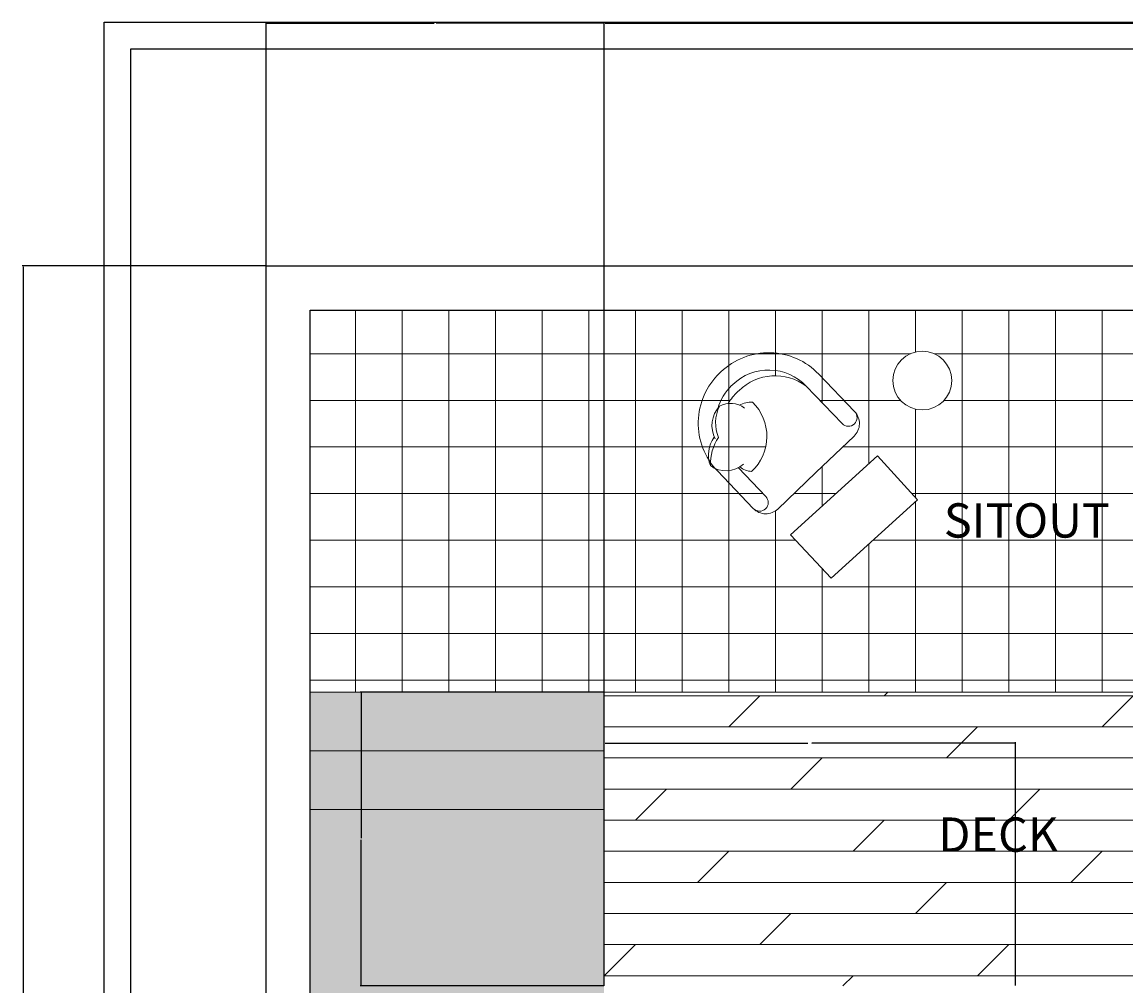
# Model space of a CAD drawing. Units: inches. Extents: x 84 to 1044, y -280 to 906.
# Tile 51 of 105: x 84 to 310, y 709 to 906. Entities that reach past the tile are written whole.
import ezdxf

# ---------------------------------------------------------------- set-up
doc = ezdxf.new("R2010")
doc.units = ezdxf.units.IN
for name, color, linetype, lineweight in [('A-ANNO-DIMS', 2, 'Continuous', 18), ('A-ANNO-TTLB', 7, 'Continuous', 25), ('A-AREA-IDEN', 7, 'Continuous', 13), ('A-FURN', 8, 'Continuous', 15), ('A-STAIRCASE', 144, 'Continuous', 18), ('C-PROP', 7, 'Continuous', 25), ('L-HRDS', 32, 'Continuous', 18)]:
    doc.layers.add(name, color=color, linetype=linetype, lineweight=lineweight)
for name, color, linetype, lineweight, true_color in [('A-FLOR-PATT', 251, 'Continuous', 9, 0x705861), ('A-FLOR-STRS-PATT', 35, 'Continuous', 9, 0x947764), ('L-PLNT-PATT', 9, 'Continuous', 9, 0xafd9aa)]:
    doc.layers.add(name, color=color, linetype=linetype, lineweight=lineweight, true_color=true_color)
doc.styles.add('1-100DIM', font='txt', dxfattribs={"height": 0.3})
doc.styles.get("Standard").update_dxf_attribs({"font": 'arial.ttf'})
doc.dimstyles.get("Standard").update_dxf_attribs({"dimtxt": 0.18, "dimasz": 0.18, "dimexe": 0.18, "dimexo": 0.0625, "dimgap": 0.09, "dimtad": 0, "dimtih": 1, "dimtoh": 1, "dimdec": 4, "dimzin": 0, "dimdsep": 46, "dimtxsty": 'Standard', "dimcen": 0.09, "dimadec": 0, "dimazin": 0, "dimtfac": 1, "dimtdec": 4, "dimtofl": 0, "dimtmove": 0, "dimatfit": 3, "dimfxl": 1, "dimtolj": 1, "dimtzin": 0, "dimarcsym": 0})

# ---------------------------------------------------------------- blocks, each defined once
blk = doc.blocks.new('*D61')
at = {"layer": 'A-ANNO-DIMS', "color": 0, "lineweight": -2, "transparency": 16777216}
for p, q in [((134.12, 856.12), (84.4, 856.12)), ((84.58, 855.94), (84.58, 367.3)), ((84.58, -121.7), (84.58, 366.94)), ((134.12, -121.88), (84.4, -121.88))]:
    blk.add_line(p, q, dxfattribs=at)
at = {"layer": 'A-ANNO-DIMS', "color": 0, "transparency": 16777216}
for points in [[(84.55, 855.94), (84.61, 855.94), (84.58, 856.12)], [(84.55, -121.7), (84.61, -121.7), (84.58, -121.88)]]:
    blk.add_solid(points, dxfattribs=at)
at = {"layer": 'Defpoints', "color": 0, "transparency": 16777216}
for p in [(84.58, 856.12), (134.18, 856.12), (134.18, -121.88)]:
    blk.add_point(p, dxfattribs=at)
at = {"layer": 'A-ANNO-DIMS', "color": 0, "transparency": 16777216, "insert": (84.58, 367.12), "char_height": 0.18, "attachment_point": 5}
blk.add_mtext('\\A1;978', dxfattribs=at)
blk = doc.blocks.new('*D62')
at = {"layer": 'A-ANNO-DIMS', "color": 0, "lineweight": -2, "transparency": 16777216}
for p, q in [((203.18, 709.18), (203.18, 905.9)), ((896.07, 400.18), (896.07, 905.9)), ((203.36, 905.72), (549.23, 905.72)), ((895.89, 905.72), (550.02, 905.72))]:
    blk.add_line(p, q, dxfattribs=at)
at = {"layer": 'A-ANNO-DIMS', "color": 0, "transparency": 16777216}
for points in [[(203.36, 905.75), (203.36, 905.69), (203.18, 905.72)], [(895.89, 905.75), (895.89, 905.69), (896.07, 905.72)]]:
    blk.add_solid(points, dxfattribs=at)
at = {"layer": 'Defpoints', "color": 0, "transparency": 16777216}
for p in [(896.07, 905.72), (203.18, 709.12), (896.07, 400.12)]:
    blk.add_point(p, dxfattribs=at)
at = {"layer": 'A-ANNO-DIMS', "color": 0, "transparency": 16777216, "insert": (549.63, 905.72), "char_height": 0.18, "attachment_point": 5}
blk.add_mtext('\\A1;692.9', dxfattribs=at)
blk = doc.blocks.new('*D64')
at = {"layer": 'A-ANNO-DIMS', "color": 0, "lineweight": -2, "transparency": 16777216}
for p, q in [((134.18, 856.18), (134.18, 905.9)), ((203.18, 709.18), (203.18, 905.9)), ((134.36, 905.72), (168.46, 905.72)), ((203, 905.72), (168.9, 905.72))]:
    blk.add_line(p, q, dxfattribs=at)
at = {"layer": 'A-ANNO-DIMS', "color": 0, "transparency": 16777216}
for points in [[(134.36, 905.75), (134.36, 905.69), (134.18, 905.72)], [(203, 905.75), (203, 905.69), (203.18, 905.72)]]:
    blk.add_solid(points, dxfattribs=at)
at = {"layer": 'Defpoints', "color": 0, "transparency": 16777216}
for p in [(203.18, 905.72), (134.18, 856.12), (203.18, 709.12)]:
    blk.add_point(p, dxfattribs=at)
at = {"layer": 'A-ANNO-DIMS', "color": 0, "transparency": 16777216, "insert": (168.68, 905.72), "char_height": 0.18, "attachment_point": 5}
blk.add_mtext('\\A1;69', dxfattribs=at)
blk = doc.blocks.new('*D77')
at = {"layer": 'A-ANNO-DIMS', "color": 0, "lineweight": -2, "transparency": 16777216}
for p, q in [((203.18, 709.18), (203.18, 758.9)), ((203.36, 758.72), (244.76, 758.72)), ((286.95, 758.72), (245.55, 758.72)), ((287.13, 709.18), (287.13, 758.9))]:
    blk.add_line(p, q, dxfattribs=at)
at = {"layer": 'A-ANNO-DIMS', "color": 0, "transparency": 16777216}
for points in [[(203.36, 758.75), (203.36, 758.69), (203.18, 758.72)], [(286.95, 758.75), (286.95, 758.69), (287.13, 758.72)]]:
    blk.add_solid(points, dxfattribs=at)
at = {"layer": 'Defpoints', "color": 0, "transparency": 16777216}
for p in [(287.13, 758.72), (203.18, 709.12), (287.13, 709.12)]:
    blk.add_point(p, dxfattribs=at)
at = {"layer": 'A-ANNO-DIMS', "color": 0, "transparency": 16777216, "insert": (245.15, 758.72), "char_height": 0.18, "attachment_point": 5}
blk.add_mtext('\\A1;83.95', dxfattribs=at)
blk = doc.blocks.new('*D78')
at = {"layer": 'A-ANNO-DIMS', "color": 0, "lineweight": -2, "transparency": 16777216}
for p, q in [((203.12, 769.12), (153.4, 769.12)), ((153.58, 768.94), (153.58, 739.3)), ((153.58, 709.3), (153.58, 738.94)), ((203.12, 709.12), (153.4, 709.12))]:
    blk.add_line(p, q, dxfattribs=at)
at = {"layer": 'A-ANNO-DIMS', "color": 0, "transparency": 16777216}
for points in [[(153.55, 768.94), (153.61, 768.94), (153.58, 769.12)], [(153.55, 709.3), (153.61, 709.3), (153.58, 709.12)]]:
    blk.add_solid(points, dxfattribs=at)
at = {"layer": 'Defpoints', "color": 0, "transparency": 16777216}
for p in [(153.58, 769.12), (203.18, 769.12), (203.18, 709.12)]:
    blk.add_point(p, dxfattribs=at)
at = {"layer": 'A-ANNO-DIMS', "color": 0, "transparency": 16777216, "insert": (153.58, 739.12), "char_height": 0.18, "attachment_point": 5}
blk.add_mtext('\\A1;60', dxfattribs=at)

msp = doc.modelspace()

# ---------------------------------------------------------------- hatches: boundary and pattern name
at = {"layer": 'A-FLOR-PATT', "transparency": 33554597}
h = msp.add_hatch(dxfattribs=at)
h.set_pattern_fill('ANSI37', color=256, scale=3, angle=45)
h.paths.add_polyline_path([(410.074, 847.12), (143.179, 847.12), (143.179, 769.12), (203.179, 769.12), (410.074, 769.12)])
h.paths.add_polyline_path([(254.313, 826.374, -0.4142136), (254.257, 823.878, -0.4142136), (251.76, 823.934), (244.439, 831.592, 0.3775004), (230.555, 830.526, 0.0765992), (228.51, 828.052, -0.127919), (230.803, 827.709, -0.1215233), (233.469, 828.328, -0.4259892), (233.291, 814.163, -0.1655406), (230.889, 815.094, -0.0168883), (230.578, 814.914), (236.189, 809.046, -0.4142136), (236.133, 806.549, -0.4142136), (233.636, 806.605, 0.4142136), (238.63, 806.493), (246.415, 813.937), (254.201, 821.381, 0.4142136)], flags=16)
h.paths.add_polyline_path([(241.241, 801.211), (258.998, 817.357), (267.168, 808.372), (249.545, 792.347)], flags=16)
h.paths.add_polyline_path([(262.121, 832.717, -1), (274.121, 832.717, -1)], flags=16)
h.paths.add_polyline_path([(315.269, 832.717, -1), (327.269, 832.717, -1)], flags=16)
h.paths.add_polyline_path([(322.221, 808.372), (330.392, 817.357), (348.148, 801.211), (339.844, 792.347)], flags=16)
h.paths.add_polyline_path([(344.951, 831.592, -0.3727189), (358.711, 830.652), (358.966, 830.408, -0.0723842), (360.879, 828.052, -0.1030417), (362.667, 827.476, -0.0234196), (363.022, 827.039, 0.1348317), (360.058, 831.805, 0.4191038)], flags=0)
h.paths.add_polyline_path([(355.753, 806.605, -0.4142136), (353.257, 806.549, -0.4142136), (353.201, 809.046), (358.811, 814.914, 0.2341585), (363.536, 814.769, 0.4037218), (362.499, 834.358, 0.4178796), (342.398, 834.032), (335.076, 826.374, 0.4142136), (335.188, 821.381), (342.974, 813.937), (350.76, 806.493, 0.4142136)], flags=16)
h = msp.add_hatch(dxfattribs=at)
h.set_pattern_fill('DOLMIT', color=256)
h.paths.add_polyline_path([(896.074, 709.12), (833.074, 709.12), (833.074, 646.12), (833.074, 574.12), (833.074, 511.12), (896.074, 511.12)])
h.paths.add_polyline_path([(386.074, 769.12), (203.179, 769.12), (203.179, 709.12), (287.127, 709.12), (359.127, 709.12), (386.074, 709.12)])
at = {"layer": 'A-FLOR-STRS-PATT', "transparency": 33554567}
h = msp.add_hatch(color=256, dxfattribs=at)
h.dxf.hatch_style = 1
h.paths.add_polyline_path([(650.074, 91.12), (638.074, 91.12), (638.074, 67.12), (455.074, 67.12), (455.074, 55.12), (650.074, 55.12)], flags=17)
h.paths.add_polyline_path([(662.074, 91.12), (650.074, 91.12), (650.074, 55.12), (455.074, 55.12), (455.074, 43.12), (662.074, 43.12)])
h.paths.add_polyline_path([(674.074, 91.12), (671.074, 91.12), (662.074, 91.12), (662.074, 43.12), (455.074, 43.12), (455.074, 31.12), (674.074, 31.12)])
h.paths.add_polyline_path([(227.179, 151.12), (203.179, 151.12), (143.179, 151.12), (143.179, 139.12), (227.179, 139.12)])
h.paths.add_polyline_path([(227.179, 139.12), (143.179, 139.12), (143.179, 127.12), (227.179, 127.12)])
h.paths.add_polyline_path([(203.179, 271.12), (143.179, 271.12), (143.179, 259.12), (203.179, 259.12)])
h.paths.add_polyline_path([(203.179, 259.12), (143.179, 259.12), (143.179, 247.12), (203.179, 247.12)])
h.paths.add_polyline_path([(203.179, 769.12), (143.179, 769.12), (143.179, 757.12), (203.179, 757.12)])
h.paths.add_polyline_path([(203.179, 757.12), (143.179, 757.12), (143.179, 745.12), (203.179, 745.12)])
h.paths.add_polyline_path([(434.074, 847.12), (422.074, 847.12), (422.074, 769.12), (434.074, 769.12)])
h.paths.add_polyline_path([(422.074, 847.12), (410.074, 847.12), (410.074, 769.12), (422.074, 769.12)])
at = {"layer": 'L-PLNT-PATT', "transparency": 33554597}
h = msp.add_hatch(color=256, dxfattribs=at)
h.dxf.hatch_style = 1
h.paths.add_polyline_path([(434.074, 769.12), (386.074, 769.12), (386.074, 709.12), (434.074, 709.12)])
h.paths.add_polyline_path([(896.074, 847.12), (434.074, 847.12), (434.074, 769.12), (434.074, 709.12), (470.074, 709.12), (506.074, 709.12), (572.074, 709.12), (608.074, 709.12), (698.074, 709.12), (770.074, 709.12), (833.074, 709.12), (896.074, 709.12)])
h.paths.add_polyline_path([(983.074, 847.12), (896.074, 847.12), (896.074, 709.12), (896.074, 547.12), (932.074, 547.12), (983.074, 547.12)])
h.paths.add_polyline_path([(983.074, 547.12), (932.074, 547.12), (932.074, 265.12), (983.074, 265.12)])
h.paths.add_polyline_path([(203.179, 646.12), (203.179, 709.12), (203.179, 745.12), (143.179, 745.12), (143.179, 271.12), (203.179, 271.12), (203.179, 274.12), (203.179, 310.12), (203.179, 574.12)])

# ---------------------------------------------------------------- linework, layer by layer
at = {"layer": 'A-ANNO-TTLB'}
for points in [[(101.1, 905.916), (1027.308, 905.916), (1027.308, -279.764), (101.1, -279.764)], [(106.576, 900.439), (1021.832, 900.439), (1021.832, -274.288), (106.576, -274.288)]]:
    msp.add_lwpolyline(points, close=True, dxfattribs=at)
at = {"layer": 'A-FURN'}
for points in [[(246.415, 813.937), (254.201, 821.381, 0.4142136), (254.313, 826.374), (246.991, 834.032, 0.4142136), (227.018, 834.481), (226.89, 834.359), (226.763, 834.237, 0.4142136), (226.314, 814.263), (233.636, 806.605, 0.4142136), (238.63, 806.493), (246.415, 813.937)], [(244.439, 831.592, 0.4142136), (229.459, 831.928), (229.331, 831.806)], [(244.439, 831.592, 0.3727189), (230.679, 830.652), (230.551, 830.53)], [(226.368, 827.039, -0.1305915), (229.203, 831.684), (229.331, 831.806)], [(244.438, 831.592), (251.76, 823.934, 0.4142136), (254.257, 823.878), (254.257, 823.878, 0.4142136), (254.313, 826.374)], [(228.51, 828.052, -0.0723842), (230.424, 830.408), (230.551, 830.53)], [(224.874, 815.352, -0.1477299), (226.507, 821.112, -0.2133428), (226.722, 827.476, -0.1786618)], [(225.824, 820.794, -0.3066635), (226.722, 827.476, -0.30633), (231.866, 827.076, 0.8728472)], [(230.889, 815.094, 0.1655406), (233.291, 814.163, 0.4259892), (233.469, 828.328, 0.1215233), (230.803, 827.709, -7.1154643)], [(231.607, 815.632, -0.3567724), (224.874, 815.352, -0.2495421), (225.653, 821.172, 9.6168803)], [(230.578, 814.914), (236.189, 809.046, -0.4142136), (236.133, 806.549), (236.133, 806.549, -0.4142136), (233.636, 806.605)]]:
    msp.add_lwpolyline(points, format="xyb", dxfattribs=at)
msp.add_lwpolyline([(258.998, 817.357), (267.168, 808.372), (249.545, 792.347), (241.241, 801.211)], close=True, dxfattribs=at)
msp.add_circle((268.121, 832.717), 6, dxfattribs=at)
at = {"layer": 'A-STAIRCASE'}
for p, q in [((203.179, 769.12), (143.179, 769.12)), ((203.179, 757.12), (143.179, 757.12)), ((203.179, 745.12), (143.179, 745.12))]:
    msp.add_line(p, q, dxfattribs=at)
at = {"layer": 'C-PROP'}
for points in [[(143.179, -121.88), (134.179, -121.88), (134.179, 856.12), (992.074, 856.12), (992.074, -121.88), (624.574, -121.88)], [(143.179, -112.88), (143.179, 847.12), (983.074, 847.12), (983.074, -112.88), (624.574, -112.88)]]:
    msp.add_lwpolyline(points, dxfattribs=at)
at = {"layer": 'L-HRDS'}
for p, q in [((203.179, 709.12), (203.179, 769.12)), ((203.179, 769.12), (434.074, 769.12))]:
    msp.add_line(p, q, dxfattribs=at)

# ---------------------------------------------------------------- texts
at = {"layer": 'A-AREA-IDEN', "char_height": 7, "attachment_point": 1, "style": '1-100DIM'}
for s, insert in [('{\\f@Malgun Gothic|b0|i0|c0|p34; SITOUT }', (270.387, 807.659)), ('{\\f@Malgun Gothic|b0|i0|c0|p34;    DECK }', (262.833, 743.516))]:
    msp.add_mtext_dynamic_manual_height_columns(s, width=51.07953, gutter_width=15.851, heights=[0], dxfattribs=dict(at, insert=insert))

# ---------------------------------------------------------------- dimensions: what is measured, and where the dimension line sits
at = {"layer": 'A-ANNO-DIMS'}
for base, p1, p2, override, picture, middle in [((203.179, 905.72), (134.179, 856.12), (203.179, 709.12), {"dimdec": 0, "dimlfac": 1, "dimrnd": 0, "dimzin": 0, "dimdsep": 46, "dimlunit": 2}, '*D64', (168.679, 905.72)), ((896.074, 905.72), (203.179, 709.12), (896.074, 400.12), {"dimdec": 1, "dimlfac": 1, "dimrnd": 0, "dimzin": 0, "dimdsep": 46, "dimlunit": 2}, '*D62', (549.627, 905.72)), ((287.127, 758.72), (203.179, 709.12), (287.127, 709.12), {"dimdec": 2, "dimlfac": 1, "dimrnd": 0, "dimzin": 0, "dimdsep": 46, "dimlunit": 2}, '*D77', (245.153, 758.72))]:
    dim = msp.add_linear_dim(base=base, p1=p1, p2=p2, dimstyle='Standard', override=override, dxfattribs=at)
    dim.commit()
    dim.dimension.update_dxf_attribs({"geometry": picture, "text_midpoint": middle})
for base, p1, p2, picture, middle in [((84.579, 856.12), (134.179, -121.88), (134.179, 856.12), '*D61', (84.579, 367.12)), ((153.579, 769.12), (203.179, 709.12), (203.179, 769.12), '*D78', (153.579, 739.12))]:
    dim = msp.add_linear_dim(base=base, p1=p1, p2=p2, angle=90, dimstyle='Standard', override={"dimdec": 0, "dimlfac": 1, "dimrnd": 0, "dimzin": 0, "dimdsep": 46, "dimlunit": 2}, dxfattribs=at)
    dim.commit()
    dim.dimension.update_dxf_attribs({"geometry": picture, "text_midpoint": middle})

doc.saveas('drawing.dxf')
